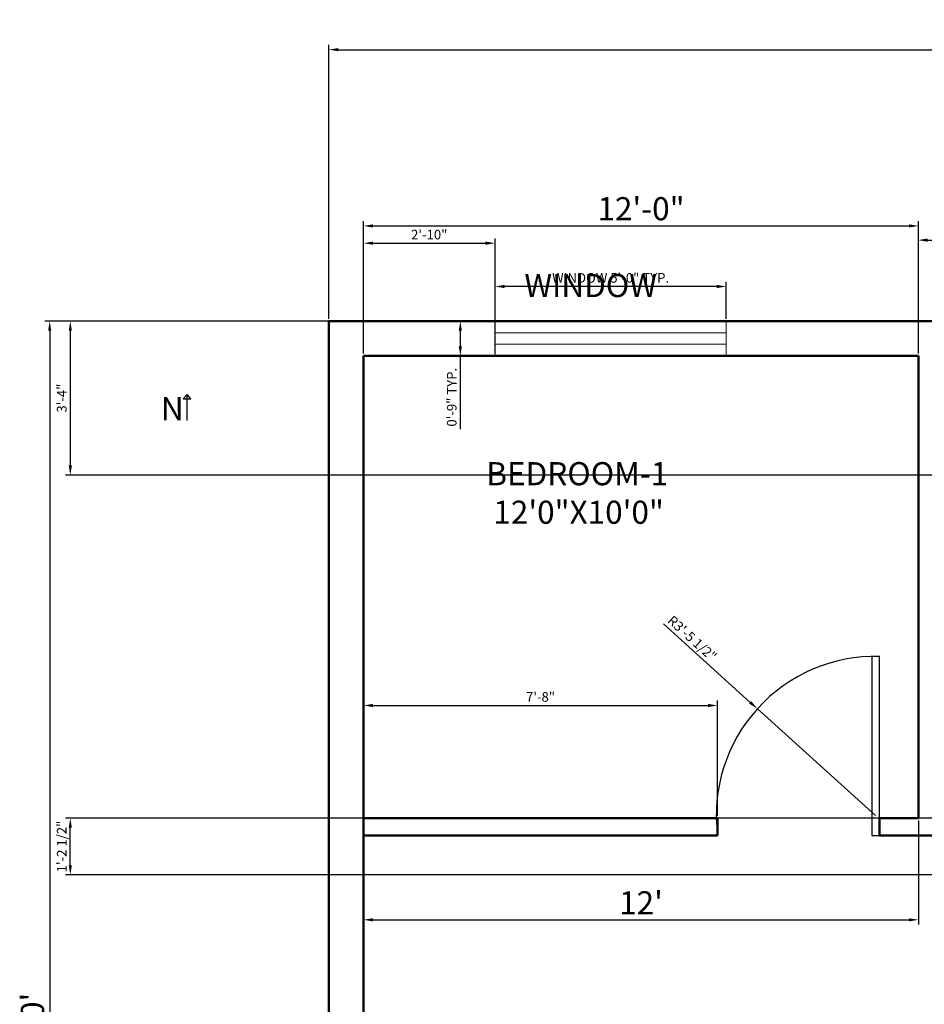
# Model space of a CAD drawing. Units: inches. Extents: x 259417 to 260009, y 246275 to 246915.
# Tile 3 of 4: x 259417 to 259652, y 246587 to 246842. Entities that reach past the tile are written whole.
import ezdxf

# ---------------------------------------------------------------- set-up
doc = ezdxf.new("R2010")
doc.units = ezdxf.units.IN
for name, color, linetype, lineweight in [('A-ANNO-DIMS', 2, 'Continuous', 18), ('A-ANNO-SYMB', 7, 'Continuous', 25), ('A-ANNO-TEXT', 7, 'Continuous', 18), ('A-AREA-IDEN', 7, 'Continuous', 25), ('A-DOOR', 3, 'Continuous', 25), ('A-GLAZ', 4, 'Continuous', 18), ('A-WALL', 7, 'Continuous', 50)]:
    doc.layers.add(name, color=color, linetype=linetype, lineweight=lineweight)
doc.styles.get("Standard").update_dxf_attribs({"font": 'arial.ttf'})
doc.dimstyles.new('ISO-25', dxfattribs={"dimtxt": 2.5, "dimasz": 2.5, "dimexe": 1.25, "dimexo": 0.625, "dimtad": 1, "dimdec": 1, "dimlunit": 3, "dimtxsty": 'Standard', "dimcen": 2.5, "dimadec": 0, "dimazin": 0, "dimtfac": 1, "dimtdec": 1, "dimtmove": 0, "dimatfit": 3, "dimfxl": 1, "dimarcsym": 0})

# ---------------------------------------------------------------- blocks, each defined once
blk = doc.blocks.new('*D8')
at = {"layer": 'A-ANNO-DIMS', "color": 0, "lineweight": -2, "transparency": 16777216}
for p, q in [((259497.59, 246764.47), (259497.59, 246835.57)), ((259500.09, 246834.32), (259975.09, 246834.32)), ((259977.59, 246764.47), (259977.59, 246835.57))]:
    blk.add_line(p, q, dxfattribs=at)
at = {"layer": 'A-ANNO-DIMS', "color": 0, "transparency": 16777216}
for points in [[(259500.09, 246834.74), (259500.09, 246833.91), (259497.59, 246834.32)], [(259975.09, 246834.74), (259975.09, 246833.91), (259977.59, 246834.32)]]:
    blk.add_solid(points, dxfattribs=at)
at = {"layer": 'Defpoints', "color": 0, "transparency": 16777216}
for p in [(259977.59, 246834.32), (259497.59, 246763.84), (259977.59, 246763.84)]:
    blk.add_point(p, dxfattribs=at)
at = {"layer": 'A-ANNO-DIMS', "color": 0, "transparency": 16777216, "insert": (259737.59, 246838.01), "char_height": 6, "attachment_point": 5}
blk.add_mtext("40'", dxfattribs=at)
blk = doc.blocks.new('*D9')
at = {"layer": 'A-ANNO-DIMS', "color": 0, "lineweight": -2, "transparency": 16777216}
for p, q in [((259496.97, 246763.84), (259423.92, 246763.84)), ((259425.17, 246761.34), (259425.17, 246406.34)), ((259496.97, 246403.84), (259423.92, 246403.84))]:
    blk.add_line(p, q, dxfattribs=at)
at = {"layer": 'A-ANNO-DIMS', "color": 0, "transparency": 16777216}
for points in [[(259424.75, 246761.34), (259425.59, 246761.34), (259425.17, 246763.84)], [(259424.75, 246406.34), (259425.59, 246406.34), (259425.17, 246403.84)]]:
    blk.add_solid(points, dxfattribs=at)
at = {"layer": 'Defpoints', "color": 0, "transparency": 16777216}
for p in [(259497.59, 246763.84), (259425.17, 246403.84), (259497.59, 246403.84)]:
    blk.add_point(p, dxfattribs=at)
at = {"layer": 'A-ANNO-DIMS', "color": 0, "transparency": 16777216, "insert": (259421.48, 246583.84), "char_height": 6, "attachment_point": 5, "rotation": 90}
blk.add_mtext("30'", dxfattribs=at)
blk = doc.blocks.new('*D11')
at = {"layer": 'A-ANNO-DIMS', "color": 0, "lineweight": -2, "transparency": 16777216}
for p, q in [((259506.59, 246755.47), (259506.59, 246789.82)), ((259509.09, 246788.57), (259648.09, 246788.57)), ((259650.59, 246755.47), (259650.59, 246789.82))]:
    blk.add_line(p, q, dxfattribs=at)
at = {"layer": 'A-ANNO-DIMS', "color": 0, "transparency": 16777216}
for points in [[(259509.09, 246788.99), (259509.09, 246788.16), (259506.59, 246788.57)], [(259648.09, 246788.99), (259648.09, 246788.16), (259650.59, 246788.57)]]:
    blk.add_solid(points, dxfattribs=at)
at = {"layer": 'Defpoints', "color": 0, "transparency": 16777216}
for p in [(259650.59, 246788.57), (259506.59, 246754.84), (259650.59, 246754.84)]:
    blk.add_point(p, dxfattribs=at)
at = {"layer": 'A-ANNO-DIMS', "color": 0, "transparency": 16777216, "insert": (259578.59, 246792.26), "char_height": 6, "attachment_point": 5}
blk.add_mtext('12\'-0"', dxfattribs=at)
blk = doc.blocks.new('*D14')
at = {"layer": 'A-ANNO-DIMS', "color": 0, "lineweight": -2, "transparency": 16777216}
for p, q in [((259650.46, 246787.95), (259650.46, 246783.64)), ((259826.09, 246787.95), (259826.09, 246783.64)), ((259652.96, 246784.89), (259823.59, 246784.89))]:
    blk.add_line(p, q, dxfattribs=at)
at = {"layer": 'A-ANNO-DIMS', "color": 0, "transparency": 16777216}
for points in [[(259652.96, 246785.31), (259652.96, 246784.47), (259650.46, 246784.89)], [(259823.59, 246785.31), (259823.59, 246784.47), (259826.09, 246784.89)]]:
    blk.add_solid(points, dxfattribs=at)
at = {"layer": 'Defpoints', "color": 0, "transparency": 16777216}
for p in [(259650.46, 246788.57), (259826.09, 246788.57), (259826.09, 246784.89)]:
    blk.add_point(p, dxfattribs=at)
at = {"layer": 'A-ANNO-DIMS', "color": 0, "transparency": 16777216, "insert": (259738.27, 246788.58), "char_height": 6, "attachment_point": 5}
blk.add_mtext('14\'-7.6"', dxfattribs=at)
blk = doc.blocks.new('*D21')
at = {"layer": 'A-ANNO-DIMS', "color": 0, "lineweight": -2, "transparency": 16777216}
for p, q in [((259650.59, 246634.22), (259650.59, 246607.2)), ((259506.59, 246629.72), (259506.59, 246607.2)), ((259509.09, 246608.45), (259648.09, 246608.45))]:
    blk.add_line(p, q, dxfattribs=at)
at = {"layer": 'A-ANNO-DIMS', "color": 0, "transparency": 16777216}
for points in [[(259509.09, 246608.86), (259509.09, 246608.03), (259506.59, 246608.45)], [(259648.09, 246608.86), (259648.09, 246608.03), (259650.59, 246608.45)]]:
    blk.add_solid(points, dxfattribs=at)
at = {"layer": 'Defpoints', "color": 0, "transparency": 16777216}
for p in [(259650.59, 246634.84), (259506.59, 246630.34), (259650.59, 246608.45)]:
    blk.add_point(p, dxfattribs=at)
at = {"layer": 'A-ANNO-DIMS', "color": 0, "transparency": 16777216, "insert": (259578.59, 246612.08), "char_height": 6, "attachment_point": 5}
blk.add_mtext("12'", dxfattribs=at)
blk = doc.blocks.new('WIN-60x9')
for p, q in [((0, 9), (0, 0)), ((60, 9), (60, 0)), ((60, 6), (0, 6)), ((60, 3), (0, 3))]:
    blk.add_line(p, q)
blk = doc.blocks.new('*D24')
at = {"layer": 'A-ANNO-DIMS', "color": 0, "lineweight": -2, "transparency": 16777216}
for p, q in [((259540.71, 246764.47), (259540.71, 246774.09)), ((259598.21, 246772.84), (259543.21, 246772.84)), ((259600.71, 246764.47), (259600.71, 246774.09))]:
    blk.add_line(p, q, dxfattribs=at)
at = {"layer": 'A-ANNO-DIMS', "color": 0, "transparency": 16777216}
for points in [[(259543.21, 246773.26), (259543.21, 246772.42), (259540.71, 246772.84)], [(259598.21, 246773.26), (259598.21, 246772.42), (259600.71, 246772.84)]]:
    blk.add_solid(points, dxfattribs=at)
at = {"layer": 'Defpoints', "color": 0, "transparency": 16777216}
for p in [(259540.71, 246772.84), (259540.71, 246763.84), (259600.71, 246763.84)]:
    blk.add_point(p, dxfattribs=at)
at = {"layer": 'A-ANNO-DIMS', "color": 0, "transparency": 16777216, "insert": (259570.71, 246774.76), "char_height": 2.5, "attachment_point": 5}
blk.add_mtext('WINDOW 5\'-0" TYP.', dxfattribs=at)
blk = doc.blocks.new('*D25')
at = {"layer": 'A-ANNO-DIMS', "color": 0, "lineweight": -2, "transparency": 16777216}
for p, q in [((259540.09, 246763.84), (259530.46, 246763.84)), ((259531.71, 246761.34), (259531.71, 246757.34)), ((259540.09, 246754.84), (259530.46, 246754.84)), ((259531.71, 246754.84), (259531.71, 246735.85))]:
    blk.add_line(p, q, dxfattribs=at)
at = {"layer": 'A-ANNO-DIMS', "color": 0, "transparency": 16777216}
for points in [[(259531.29, 246761.34), (259532.13, 246761.34), (259531.71, 246763.84)], [(259531.29, 246757.34), (259532.13, 246757.34), (259531.71, 246754.84)]]:
    blk.add_solid(points, dxfattribs=at)
at = {"layer": 'Defpoints', "color": 0, "transparency": 16777216}
for p in [(259540.71, 246763.84), (259531.71, 246754.84), (259540.71, 246754.84)]:
    blk.add_point(p, dxfattribs=at)
at = {"layer": 'A-ANNO-DIMS', "color": 0, "transparency": 16777216, "insert": (259529.81, 246744.1), "char_height": 2.5, "attachment_point": 5, "rotation": 90}
blk.add_mtext('0\'-9" TYP.', dxfattribs=at)
blk = doc.blocks.new('*D34')
at = {"layer": 'A-ANNO-DIMS', "color": 0, "lineweight": -2, "transparency": 16777216}
for p, q in [((259506.59, 246755.47), (259506.59, 246785.34)), ((259540.71, 246755.47), (259540.71, 246785.34)), ((259509.09, 246784.09), (259538.21, 246784.09))]:
    blk.add_line(p, q, dxfattribs=at)
at = {"layer": 'A-ANNO-DIMS', "color": 0, "transparency": 16777216}
for points in [[(259509.09, 246784.51), (259509.09, 246783.67), (259506.59, 246784.09)], [(259538.21, 246784.51), (259538.21, 246783.67), (259540.71, 246784.09)]]:
    blk.add_solid(points, dxfattribs=at)
at = {"layer": 'Defpoints', "color": 0, "transparency": 16777216}
for p in [(259540.71, 246784.09), (259506.59, 246754.84), (259540.71, 246754.84)]:
    blk.add_point(p, dxfattribs=at)
at = {"layer": 'A-ANNO-DIMS', "color": 0, "transparency": 16777216, "insert": (259523.65, 246785.99), "char_height": 2.5, "attachment_point": 5}
blk.add_mtext('2\'-10"', dxfattribs=at)
blk = doc.blocks.new('*D42')
at = {"layer": 'A-ANNO-DIMS', "color": 0, "lineweight": -2, "transparency": 16777216}
for p, q in [((259825.47, 246763.84), (259429.27, 246763.84)), ((259430.52, 246761.34), (259430.52, 246726.39)), ((259825.47, 246723.89), (259429.27, 246723.89))]:
    blk.add_line(p, q, dxfattribs=at)
at = {"layer": 'A-ANNO-DIMS', "color": 0, "transparency": 16777216}
for points in [[(259430.11, 246761.34), (259430.94, 246761.34), (259430.52, 246763.84)], [(259430.11, 246726.39), (259430.94, 246726.39), (259430.52, 246723.89)]]:
    blk.add_solid(points, dxfattribs=at)
at = {"layer": 'Defpoints', "color": 0, "transparency": 16777216}
for p in [(259826.09, 246763.84), (259430.52, 246723.89), (259826.09, 246723.89)]:
    blk.add_point(p, dxfattribs=at)
at = {"layer": 'A-ANNO-DIMS', "color": 0, "transparency": 16777216, "insert": (259428.62, 246743.87), "char_height": 2.5, "attachment_point": 5, "rotation": 90}
blk.add_mtext('3\'-4"', dxfattribs=at)
blk = doc.blocks.new('*D50')
at = {"layer": 'A-ANNO-DIMS', "color": 0, "lineweight": -2, "transparency": 16777216}
for p, q in [((259506.59, 246635.47), (259506.59, 246665.34)), ((259598.45, 246635.47), (259598.45, 246665.34)), ((259509.09, 246664.09), (259595.95, 246664.09))]:
    blk.add_line(p, q, dxfattribs=at)
at = {"layer": 'A-ANNO-DIMS', "color": 0, "transparency": 16777216}
for points in [[(259509.09, 246664.51), (259509.09, 246663.67), (259506.59, 246664.09)], [(259595.95, 246664.51), (259595.95, 246663.67), (259598.45, 246664.09)]]:
    blk.add_solid(points, dxfattribs=at)
at = {"layer": 'Defpoints', "color": 0, "transparency": 16777216}
for p in [(259598.45, 246664.09), (259506.59, 246634.84), (259598.45, 246634.84)]:
    blk.add_point(p, dxfattribs=at)
at = {"layer": 'A-ANNO-DIMS', "color": 0, "transparency": 16777216, "insert": (259552.52, 246665.99), "char_height": 2.5, "attachment_point": 5}
blk.add_mtext('7\'-8"', dxfattribs=at)
blk = doc.blocks.new('*D55')
at = {"layer": 'A-ANNO-DIMS', "color": 0, "lineweight": -2, "transparency": 16777216}
for p, q in [((259889.08, 246634.84), (259429.27, 246634.84)), ((259430.52, 246622.6), (259430.52, 246632.34)), ((259889.08, 246620.1), (259429.27, 246620.1))]:
    blk.add_line(p, q, dxfattribs=at)
at = {"layer": 'A-ANNO-DIMS', "color": 0, "transparency": 16777216}
for points in [[(259430.11, 246632.34), (259430.94, 246632.34), (259430.52, 246634.84)], [(259430.11, 246622.6), (259430.94, 246622.6), (259430.52, 246620.1)]]:
    blk.add_solid(points, dxfattribs=at)
at = {"layer": 'Defpoints', "color": 0, "transparency": 16777216}
for p in [(259430.52, 246634.84), (259889.71, 246634.84), (259889.71, 246620.1)]:
    blk.add_point(p, dxfattribs=at)
at = {"layer": 'A-ANNO-DIMS', "color": 0, "transparency": 16777216, "insert": (259428.61, 246627.47), "char_height": 2.5, "attachment_point": 5, "rotation": 90}
blk.add_mtext('1\'-2 1/2"', dxfattribs=at)
blk = doc.blocks.new('*D66')
at = {"layer": 'A-ANNO-DIMS', "color": 0, "lineweight": -2, "transparency": 16777216}
for p, q in [((259584.4, 246685.25), (259606.92, 246664.9)), ((259639.45, 246635.53), (259608.78, 246663.23))]:
    blk.add_line(p, q, dxfattribs=at)
at = {"layer": 'A-ANNO-DIMS', "color": 0, "transparency": 16777216}
blk.add_solid([(259607.2, 246665.21), (259606.64, 246664.59), (259608.78, 246663.23)], dxfattribs=at)
at = {"layer": 'Defpoints', "color": 0, "transparency": 16777216}
for p in [(259608.78, 246663.23), (259639.45, 246635.53)]:
    blk.add_point(p, dxfattribs=at)
at = {"layer": 'A-ANNO-DIMS', "color": 0, "transparency": 16777216, "insert": (259591.66, 246681.27), "char_height": 2.5, "attachment_point": 5, "rotation": 317.9108}
blk.add_mtext('R3\'-5 1/2"', dxfattribs=at)

msp = doc.modelspace()

# ---------------------------------------------------------------- linework, layer by layer
at = {"layer": 'A-ANNO-SYMB'}
for p, q in [((259460.84, 246744.83), (259459.77, 246743.72)), ((259460.84, 246738.09), (259460.84, 246744.83)), ((259461.83, 246743.72), (259460.84, 246744.83)), ((259459.77, 246743.72), (259461.83, 246743.72))]:
    msp.add_line(p, q, dxfattribs=at)
at = {"layer": 'A-DOOR'}
for p, q in [((259640.45, 246676.84), (259638.45, 246676.84)), ((259638.45, 246676.84), (259638.45, 246630.34)), ((259640.45, 246634.84), (259640.45, 246676.84)), ((259638.45, 246630.34), (259640.45, 246630.34))]:
    msp.add_line(p, q, dxfattribs=at)
msp.add_arc((259639.45, 246635.53), 41.33, 88.6135, 187.2082, dxfattribs=at)
at = {"layer": 'A-WALL'}
for p, q in [((259497.59, 246763.84), (259655.09, 246763.84)), ((259497.59, 246403.84), (259497.59, 246763.84)), ((259506.59, 246754.84), (259650.59, 246754.84)), ((259506.59, 246412.84), (259506.59, 246754.84)), ((259650.59, 246634.84), (259650.59, 246754.84)), ((259506.59, 246634.84), (259598.45, 246634.84)), ((259598.45, 246634.84), (259598.45, 246630.34)), ((259640.45, 246634.84), (259640.45, 246630.34)), ((259640.45, 246634.84), (259650.59, 246634.84)), ((259506.59, 246630.34), (259598.45, 246630.34)), ((259640.45, 246630.34), (259776.94, 246630.34))]:
    msp.add_line(p, q, dxfattribs=at)

# ---------------------------------------------------------------- block references
at = {"layer": 'A-GLAZ', "rotation": 180}
msp.add_blockref('WIN-60x9', (259600.71, 246763.84), dxfattribs=at)

# ---------------------------------------------------------------- texts
at = {"layer": 'A-ANNO-SYMB', "insert": (259454.02, 246744.12), "char_height": 6, "attachment_point": 1}
msp.add_mtext_dynamic_manual_height_columns('N', width=1.3672, gutter_width=12.5, heights=[0], dxfattribs=at)
at = {"layer": 'A-ANNO-TEXT', "insert": (259539.16, 246776.09), "char_height": 6, "attachment_point": 1}
msp.add_mtext_dynamic_manual_height_columns('     WINDOW', width=60.426, gutter_width=12.5, heights=[18.16], dxfattribs=at)
at = {"layer": 'A-AREA-IDEN', "insert": (259532.94, 246727.25), "char_height": 6, "attachment_point": 1}
msp.add_mtext_dynamic_manual_height_columns('   BEDROOM-1\\P    12\'0"X10\'0"', width=60.426, gutter_width=12.5, heights=[18.16], dxfattribs=at)

# ---------------------------------------------------------------- dimensions: what is measured, and where the dimension line sits
at = {"layer": 'A-ANNO-DIMS'}
for base, p1, p2, override, picture, middle in [((259977.59, 246834.32), (259497.59, 246763.84), (259977.59, 246763.84), {"dimtxt": 6, "dimclrd": 0, "dimclre": 0, "dimclrt": 0}, '*D8', (259737.59, 246838.01)), ((259826.09, 246784.89), (259650.46, 246788.57), (259826.09, 246788.57), {"dimtxt": 6, "dimclrd": 0, "dimclre": 0, "dimclrt": 0}, '*D14', (259738.27, 246788.58)), ((259598.45, 246664.09), (259506.59, 246634.84), (259598.45, 246634.84), {"dimdec": 1, "dimlfac": 1, "dimrnd": 0, "dimzin": 1, "dimdsep": 46, "dimlunit": 4, "dimfrac": 2}, '*D50', (259552.52, 246665.99)), ((259650.59, 246608.45), (259506.59, 246630.34), (259650.59, 246634.84), {"dimtxt": 6, "dimclrd": 0, "dimclre": 0, "dimclrt": 0}, '*D21', (259578.59, 246612.08))]:
    dim = msp.add_linear_dim(base=base, p1=p1, p2=p2, dimstyle='ISO-25', override=override, dxfattribs=at)
    dim.commit()
    dim.dimension.update_dxf_attribs({"geometry": picture, "text_midpoint": middle})
dim = msp.add_linear_dim(base=(259650.59, 246788.57), p1=(259506.59, 246754.84), p2=(259650.59, 246754.84), text='<>-0"', dimstyle='ISO-25', override={"dimtxt": 6, "dimclrd": 0, "dimclre": 0, "dimclrt": 0}, dxfattribs=at)
dim.commit()
dim.dimension.update_dxf_attribs({"geometry": '*D11', "text_midpoint": (259578.59, 246792.26)})
for base, p1, p2, angle, override, picture, middle in [((259540.71, 246784.09), (259506.59, 246754.84), (259540.71, 246754.84), 0, {"dimdec": 1, "dimlfac": 1, "dimrnd": 0, "dimzin": 1, "dimdsep": 46, "dimlunit": 4, "dimfrac": 2}, '*D34', (259523.65, 246785.99)), ((259425.17, 246403.84), (259497.59, 246763.84), (259497.59, 246403.84), 90, {"dimtxt": 6, "dimclrd": 0, "dimclre": 0, "dimclrt": 0}, '*D9', (259421.48, 246583.84)), ((259430.5233, 246723.8897), (259826.0916, 246763.8406), (259826.0916, 246723.8897), 90, {"dimdec": 1, "dimlfac": 1, "dimrnd": 0, "dimzin": 1, "dimdsep": 46, "dimlunit": 4, "dimfrac": 2}, '*D42', (259428.621, 246743.8652)), ((259430.52, 246634.84), (259889.71, 246620.1), (259889.71, 246634.84), 90, {"dimdec": 1, "dimlfac": 1, "dimrnd": 0, "dimzin": 1, "dimdsep": 46, "dimlunit": 4, "dimfrac": 2}, '*D55', (259428.61, 246627.47))]:
    dim = msp.add_linear_dim(base=base, p1=p1, p2=p2, angle=angle, dimstyle='ISO-25', override=override, dxfattribs=at)
    dim.commit()
    dim.dimension.update_dxf_attribs({"geometry": picture, "text_midpoint": middle})
for base, p1, p2, angle, text, picture, middle in [((259540.71, 246772.84), (259600.71, 246763.84), (259540.71, 246763.84), 180, 'WINDOW <> TYP.', '*D24', (259570.71, 246774.76)), ((259531.71, 246754.84), (259540.71, 246763.84), (259540.71, 246754.84), 270, '<> TYP.', '*D25', (259529.81, 246744.1))]:
    dim = msp.add_linear_dim(base=base, p1=p1, p2=p2, angle=angle, text=text, dimstyle='ISO-25', override={"dimdec": 1, "dimlfac": 1, "dimrnd": 0, "dimzin": 1, "dimdsep": 46, "dimlunit": 4, "dimfrac": 2}, dxfattribs=at)
    dim.commit()
    dim.dimension.update_dxf_attribs({"geometry": picture, "text_midpoint": middle})
dim = msp.add_radius_dim(center=(259639.45, 246635.53), mpoint=(259608.78, 246663.23), dimstyle='ISO-25', override={"dimdec": 1, "dimlfac": 1, "dimrnd": 0, "dimzin": 1, "dimdsep": 46, "dimlunit": 4, "dimfrac": 2}, dxfattribs=at)
dim.commit()
dim.dimension.update_dxf_attribs({"geometry": '*D66', "text_midpoint": (259590.38, 246679.85), "dimtype": 164})

doc.saveas('drawing.dxf')
